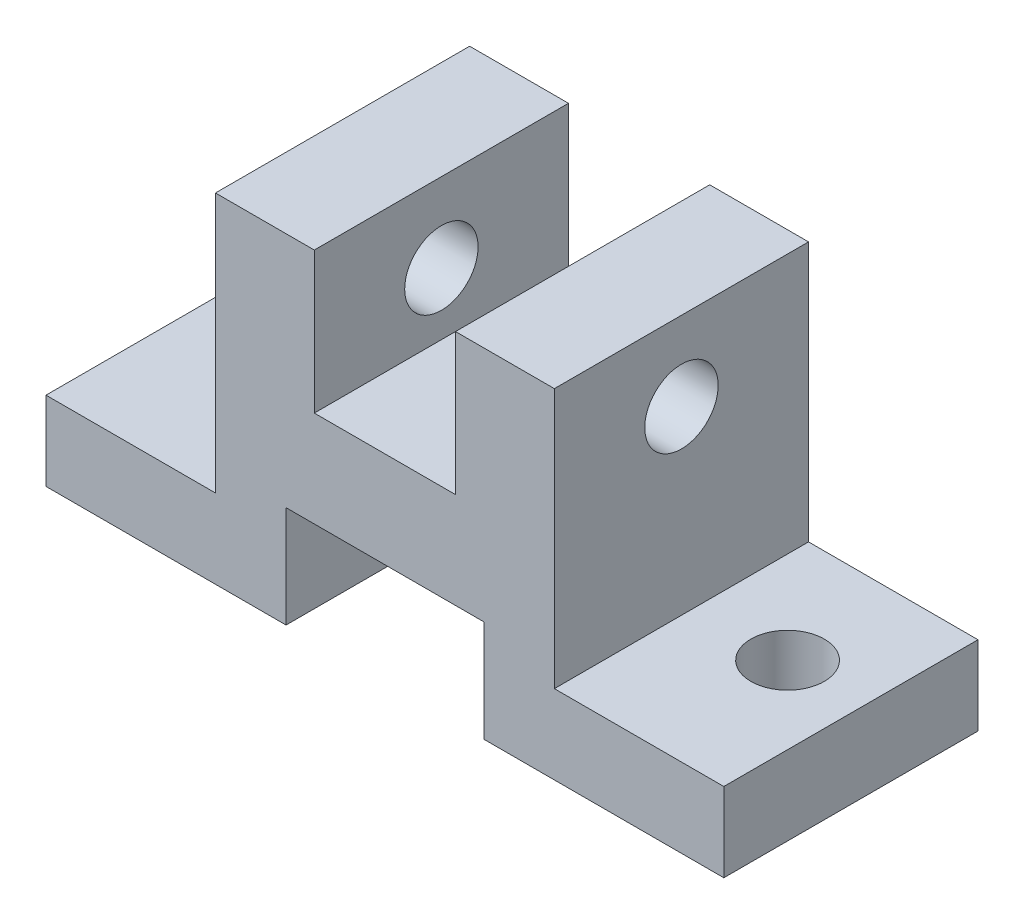
ISO-10303-21;
HEADER;
FILE_DESCRIPTION(('STEP AP214'),'2;1');
FILE_NAME('part.step','',(''),(''),'','','');
FILE_SCHEMA(('AUTOMOTIVE_DESIGN { 1 0 10303 214 1 1 1 1 }'));
ENDSEC;
DATA;
#1=APPLICATION_CONTEXT('core data for automotive mechanical design processes');
#2=APPLICATION_PROTOCOL_DEFINITION('international standard','automotive_design',2000,#1);
#3=PRODUCT_CONTEXT('',#1,'mechanical');
#4=PRODUCT('Part','Part','',(#3));
#5=PRODUCT_RELATED_PRODUCT_CATEGORY('part','',(#4));
#6=PRODUCT_DEFINITION_FORMATION('','',#4);
#7=PRODUCT_DEFINITION_CONTEXT('part definition',#1,'design');
#8=PRODUCT_DEFINITION('design','',#6,#7);
#9=PRODUCT_DEFINITION_SHAPE('','',#8);
#10=(LENGTH_UNIT() NAMED_UNIT(*) SI_UNIT(.MILLI.,.METRE.));
#11=(NAMED_UNIT(*) PLANE_ANGLE_UNIT() SI_UNIT($,.RADIAN.));
#12=(NAMED_UNIT(*) SI_UNIT($,.STERADIAN.) SOLID_ANGLE_UNIT());
#13=UNCERTAINTY_MEASURE_WITH_UNIT(LENGTH_MEASURE(1.E-05),#10,'distance_accuracy_value','');
#14=(GEOMETRIC_REPRESENTATION_CONTEXT(3) GLOBAL_UNCERTAINTY_ASSIGNED_CONTEXT((#13)) GLOBAL_UNIT_ASSIGNED_CONTEXT((#10,
#11,#12)) REPRESENTATION_CONTEXT('',''));
#15=CARTESIAN_POINT('',(0.,0.,0.));
#16=DIRECTION('',(0.,0.,1.));
#17=DIRECTION('',(1.,0.,0.));
#18=AXIS2_PLACEMENT_3D('',#15,#16,#17);
#19=CARTESIAN_POINT('',(0.,14.,45.));
#20=DIRECTION('',(1.,0.,0.));
#21=DIRECTION('',(0.,0.,-1.));
#22=AXIS2_PLACEMENT_3D('',#19,#20,#21);
#23=PLANE('',#22);
#24=DIRECTION('',(0.,-1.,0.));
#25=VECTOR('',#24,1.);
#26=CARTESIAN_POINT('',(0.,14.,0.));
#27=LINE('',#26,#25);
#28=CARTESIAN_POINT('',(0.,14.,0.));
#29=VERTEX_POINT('',#28);
#30=CARTESIAN_POINT('',(0.,0.,0.));
#31=VERTEX_POINT('',#30);
#32=EDGE_CURVE('E186',#29,#31,#27,.T.);
#33=ORIENTED_EDGE('',*,*,#32,.T.);
#34=DIRECTION('',(0.,0.,-1.));
#35=VECTOR('',#34,1.);
#36=CARTESIAN_POINT('',(0.,0.,45.));
#37=LINE('',#36,#35);
#38=CARTESIAN_POINT('',(0.,0.,45.));
#39=VERTEX_POINT('',#38);
#40=EDGE_CURVE('E11',#39,#31,#37,.T.);
#41=ORIENTED_EDGE('',*,*,#40,.F.);
#42=DIRECTION('',(0.,-1.,0.));
#43=VECTOR('',#42,1.);
#44=CARTESIAN_POINT('',(0.,14.,45.));
#45=LINE('',#44,#43);
#46=CARTESIAN_POINT('',(0.,14.,45.));
#47=VERTEX_POINT('',#46);
#48=EDGE_CURVE('E219',#47,#39,#45,.T.);
#49=ORIENTED_EDGE('',*,*,#48,.F.);
#50=DIRECTION('',(0.,0.,-1.));
#51=VECTOR('',#50,1.);
#52=CARTESIAN_POINT('',(0.,14.,45.));
#53=LINE('',#52,#51);
#54=EDGE_CURVE('E183',#47,#29,#53,.T.);
#55=ORIENTED_EDGE('',*,*,#54,.T.);
#56=EDGE_LOOP('',(#33,#41,#49,#55));
#57=FACE_BOUND('',#56,.T.);
#58=ADVANCED_FACE('F44',(#57),#23,.F.);
#59=CARTESIAN_POINT('',(0.,0.,45.));
#60=DIRECTION('',(0.,1.,0.));
#61=DIRECTION('',(0.,0.,1.));
#62=AXIS2_PLACEMENT_3D('',#59,#60,#61);
#63=PLANE('',#62);
#64=CARTESIAN_POINT('',(14.9196566145719,0.,20.));
#65=DIRECTION('',(0.,1.,0.));
#66=DIRECTION('',(0.,0.,1.));
#67=AXIS2_PLACEMENT_3D('',#64,#65,#66);
#68=CIRCLE('',#67,6.5);
#69=CARTESIAN_POINT('',(14.9196566145719,0.,26.5));
#70=VERTEX_POINT('',#69);
#71=EDGE_CURVE('E586',#70,#70,#68,.T.);
#72=ORIENTED_EDGE('',*,*,#71,.T.);
#73=EDGE_LOOP('',(#72));
#74=FACE_BOUND('',#73,.T.);
#75=DIRECTION('',(1.,0.,0.));
#76=VECTOR('',#75,1.);
#77=CARTESIAN_POINT('',(0.,0.,0.));
#78=LINE('',#77,#76);
#79=CARTESIAN_POINT('',(42.5,0.,0.));
#80=VERTEX_POINT('',#79);
#81=EDGE_CURVE('E195',#31,#80,#78,.T.);
#82=ORIENTED_EDGE('',*,*,#81,.T.);
#83=DIRECTION('',(0.,0.,-1.));
#84=VECTOR('',#83,1.);
#85=CARTESIAN_POINT('',(42.5,0.,45.));
#86=LINE('',#85,#84);
#87=CARTESIAN_POINT('',(42.5,0.,45.));
#88=VERTEX_POINT('',#87);
#89=EDGE_CURVE('E52',#88,#80,#86,.T.);
#90=ORIENTED_EDGE('',*,*,#89,.F.);
#91=DIRECTION('',(1.,0.,0.));
#92=VECTOR('',#91,1.);
#93=CARTESIAN_POINT('',(0.,0.,45.));
#94=LINE('',#93,#92);
#95=EDGE_CURVE('E126',#39,#88,#94,.T.);
#96=ORIENTED_EDGE('',*,*,#95,.F.);
#97=ORIENTED_EDGE('',*,*,#40,.T.);
#98=EDGE_LOOP('',(#82,#90,#96,#97));
#99=FACE_BOUND('',#98,.T.);
#100=ADVANCED_FACE('F321',(#74,#99),#63,.F.);
#101=CARTESIAN_POINT('',(42.5,0.,45.));
#102=DIRECTION('',(-1.,0.,0.));
#103=DIRECTION('',(0.,0.,1.));
#104=AXIS2_PLACEMENT_3D('',#101,#102,#103);
#105=PLANE('',#104);
#106=DIRECTION('',(0.,1.,0.));
#107=VECTOR('',#106,1.);
#108=CARTESIAN_POINT('',(42.5,0.,0.));
#109=LINE('',#108,#107);
#110=CARTESIAN_POINT('',(42.5,18.,0.));
#111=VERTEX_POINT('',#110);
#112=EDGE_CURVE('E192',#80,#111,#109,.T.);
#113=ORIENTED_EDGE('',*,*,#112,.T.);
#114=DIRECTION('',(0.,0.,-1.));
#115=VECTOR('',#114,1.);
#116=CARTESIAN_POINT('',(42.5,18.,45.));
#117=LINE('',#116,#115);
#118=CARTESIAN_POINT('',(42.5,18.,45.));
#119=VERTEX_POINT('',#118);
#120=EDGE_CURVE('E253',#119,#111,#117,.T.);
#121=ORIENTED_EDGE('',*,*,#120,.F.);
#122=DIRECTION('',(0.,1.,0.));
#123=VECTOR('',#122,1.);
#124=CARTESIAN_POINT('',(42.5,0.,45.));
#125=LINE('',#124,#123);
#126=EDGE_CURVE('E259',#88,#119,#125,.T.);
#127=ORIENTED_EDGE('',*,*,#126,.F.);
#128=ORIENTED_EDGE('',*,*,#89,.T.);
#129=EDGE_LOOP('',(#113,#121,#127,#128));
#130=FACE_BOUND('',#129,.T.);
#131=ADVANCED_FACE('F260',(#130),#105,.F.);
#132=CARTESIAN_POINT('',(42.5,18.,45.));
#133=DIRECTION('',(0.,1.,0.));
#134=DIRECTION('',(0.,0.,1.));
#135=AXIS2_PLACEMENT_3D('',#132,#133,#134);
#136=PLANE('',#135);
#137=DIRECTION('',(1.,0.,0.));
#138=VECTOR('',#137,1.);
#139=CARTESIAN_POINT('',(42.5,18.,0.));
#140=LINE('',#139,#138);
#141=CARTESIAN_POINT('',(77.5,18.,0.));
#142=VERTEX_POINT('',#141);
#143=EDGE_CURVE('E197',#111,#142,#140,.T.);
#144=ORIENTED_EDGE('',*,*,#143,.T.);
#145=DIRECTION('',(0.,0.,-1.));
#146=VECTOR('',#145,1.);
#147=CARTESIAN_POINT('',(77.5,18.,45.));
#148=LINE('',#147,#146);
#149=CARTESIAN_POINT('',(77.5,18.,45.));
#150=VERTEX_POINT('',#149);
#151=EDGE_CURVE('E246',#150,#142,#148,.T.);
#152=ORIENTED_EDGE('',*,*,#151,.F.);
#153=DIRECTION('',(1.,0.,0.));
#154=VECTOR('',#153,1.);
#155=CARTESIAN_POINT('',(42.5,18.,45.));
#156=LINE('',#155,#154);
#157=EDGE_CURVE('E280',#119,#150,#156,.T.);
#158=ORIENTED_EDGE('',*,*,#157,.F.);
#159=ORIENTED_EDGE('',*,*,#120,.T.);
#160=EDGE_LOOP('',(#144,#152,#158,#159));
#161=FACE_BOUND('',#160,.T.);
#162=ADVANCED_FACE('F268',(#161),#136,.F.);
#163=CARTESIAN_POINT('',(77.5,18.,45.));
#164=DIRECTION('',(1.,0.,0.));
#165=DIRECTION('',(0.,0.,-1.));
#166=AXIS2_PLACEMENT_3D('',#163,#164,#165);
#167=PLANE('',#166);
#168=DIRECTION('',(0.,-1.,0.));
#169=VECTOR('',#168,1.);
#170=CARTESIAN_POINT('',(77.5,18.,0.));
#171=LINE('',#170,#169);
#172=CARTESIAN_POINT('',(77.5,0.,0.));
#173=VERTEX_POINT('',#172);
#174=EDGE_CURVE('E200',#142,#173,#171,.T.);
#175=ORIENTED_EDGE('',*,*,#174,.T.);
#176=DIRECTION('',(0.,0.,-1.));
#177=VECTOR('',#176,1.);
#178=CARTESIAN_POINT('',(77.5,0.,45.));
#179=LINE('',#178,#177);
#180=CARTESIAN_POINT('',(77.5,0.,45.));
#181=VERTEX_POINT('',#180);
#182=EDGE_CURVE('E243',#181,#173,#179,.T.);
#183=ORIENTED_EDGE('',*,*,#182,.F.);
#184=DIRECTION('',(0.,-1.,0.));
#185=VECTOR('',#184,1.);
#186=CARTESIAN_POINT('',(77.5,18.,45.));
#187=LINE('',#186,#185);
#188=EDGE_CURVE('E273',#150,#181,#187,.T.);
#189=ORIENTED_EDGE('',*,*,#188,.F.);
#190=ORIENTED_EDGE('',*,*,#151,.T.);
#191=EDGE_LOOP('',(#175,#183,#189,#190));
#192=FACE_BOUND('',#191,.T.);
#193=ADVANCED_FACE('F275',(#192),#167,.F.);
#194=CARTESIAN_POINT('',(77.5,0.,45.));
#195=DIRECTION('',(0.,1.,0.));
#196=DIRECTION('',(0.,0.,1.));
#197=AXIS2_PLACEMENT_3D('',#194,#195,#196);
#198=PLANE('',#197);
#199=CARTESIAN_POINT('',(106.287852583252,0.,20.));
#200=DIRECTION('',(0.,1.,0.));
#201=DIRECTION('',(0.,0.,1.));
#202=AXIS2_PLACEMENT_3D('',#199,#200,#201);
#203=CIRCLE('',#202,6.5);
#204=CARTESIAN_POINT('',(106.287852583252,0.,26.5));
#205=VERTEX_POINT('',#204);
#206=EDGE_CURVE('E577',#205,#205,#203,.T.);
#207=ORIENTED_EDGE('',*,*,#206,.T.);
#208=EDGE_LOOP('',(#207));
#209=FACE_BOUND('',#208,.T.);
#210=DIRECTION('',(1.,0.,0.));
#211=VECTOR('',#210,1.);
#212=CARTESIAN_POINT('',(77.5,0.,0.));
#213=LINE('',#212,#211);
#214=CARTESIAN_POINT('',(120.,0.,0.));
#215=VERTEX_POINT('',#214);
#216=EDGE_CURVE('E203',#173,#215,#213,.T.);
#217=ORIENTED_EDGE('',*,*,#216,.T.);
#218=DIRECTION('',(0.,0.,-1.));
#219=VECTOR('',#218,1.);
#220=CARTESIAN_POINT('',(120.,0.,45.));
#221=LINE('',#220,#219);
#222=CARTESIAN_POINT('',(120.,0.,45.));
#223=VERTEX_POINT('',#222);
#224=EDGE_CURVE('E244',#223,#215,#221,.T.);
#225=ORIENTED_EDGE('',*,*,#224,.F.);
#226=DIRECTION('',(1.,0.,0.));
#227=VECTOR('',#226,1.);
#228=CARTESIAN_POINT('',(77.5,0.,45.));
#229=LINE('',#228,#227);
#230=EDGE_CURVE('E277',#181,#223,#229,.T.);
#231=ORIENTED_EDGE('',*,*,#230,.F.);
#232=ORIENTED_EDGE('',*,*,#182,.T.);
#233=EDGE_LOOP('',(#217,#225,#231,#232));
#234=FACE_BOUND('',#233,.T.);
#235=ADVANCED_FACE('F337',(#209,#234),#198,.F.);
#236=CARTESIAN_POINT('',(120.,0.,45.));
#237=DIRECTION('',(-1.,0.,0.));
#238=DIRECTION('',(0.,0.,1.));
#239=AXIS2_PLACEMENT_3D('',#236,#237,#238);
#240=PLANE('',#239);
#241=DIRECTION('',(0.,1.,0.));
#242=VECTOR('',#241,1.);
#243=CARTESIAN_POINT('',(120.,0.,0.));
#244=LINE('',#243,#242);
#245=CARTESIAN_POINT('',(120.,14.,0.));
#246=VERTEX_POINT('',#245);
#247=EDGE_CURVE('E201',#215,#246,#244,.T.);
#248=ORIENTED_EDGE('',*,*,#247,.T.);
#249=DIRECTION('',(0.,0.,-1.));
#250=VECTOR('',#249,1.);
#251=CARTESIAN_POINT('',(120.,14.,45.));
#252=LINE('',#251,#250);
#253=CARTESIAN_POINT('',(120.,14.,45.));
#254=VERTEX_POINT('',#253);
#255=EDGE_CURVE('E239',#254,#246,#252,.T.);
#256=ORIENTED_EDGE('',*,*,#255,.F.);
#257=DIRECTION('',(0.,1.,0.));
#258=VECTOR('',#257,1.);
#259=CARTESIAN_POINT('',(120.,0.,45.));
#260=LINE('',#259,#258);
#261=EDGE_CURVE('E276',#223,#254,#260,.T.);
#262=ORIENTED_EDGE('',*,*,#261,.F.);
#263=ORIENTED_EDGE('',*,*,#224,.T.);
#264=EDGE_LOOP('',(#248,#256,#262,#263));
#265=FACE_BOUND('',#264,.T.);
#266=ADVANCED_FACE('F336',(#265),#240,.F.);
#267=CARTESIAN_POINT('',(120.,14.,45.));
#268=DIRECTION('',(0.,-1.,0.));
#269=DIRECTION('',(0.,0.,-1.));
#270=AXIS2_PLACEMENT_3D('',#267,#268,#269);
#271=PLANE('',#270);
#272=CARTESIAN_POINT('',(106.287852583252,14.,20.));
#273=DIRECTION('',(0.,1.,0.));
#274=DIRECTION('',(0.,0.,1.));
#275=AXIS2_PLACEMENT_3D('',#272,#273,#274);
#276=CIRCLE('',#275,6.5);
#277=CARTESIAN_POINT('',(106.287852583252,14.,26.5));
#278=VERTEX_POINT('',#277);
#279=EDGE_CURVE('E581',#278,#278,#276,.T.);
#280=ORIENTED_EDGE('',*,*,#279,.F.);
#281=EDGE_LOOP('',(#280));
#282=FACE_BOUND('',#281,.T.);
#283=DIRECTION('',(-1.,0.,0.));
#284=VECTOR('',#283,1.);
#285=CARTESIAN_POINT('',(120.,14.,0.));
#286=LINE('',#285,#284);
#287=CARTESIAN_POINT('',(90.,14.,0.));
#288=VERTEX_POINT('',#287);
#289=EDGE_CURVE('E202',#246,#288,#286,.T.);
#290=ORIENTED_EDGE('',*,*,#289,.T.);
#291=DIRECTION('',(0.,0.,-1.));
#292=VECTOR('',#291,1.);
#293=CARTESIAN_POINT('',(90.,14.,45.));
#294=LINE('',#293,#292);
#295=CARTESIAN_POINT('',(90.,14.,45.));
#296=VERTEX_POINT('',#295);
#297=EDGE_CURVE('E237',#296,#288,#294,.T.);
#298=ORIENTED_EDGE('',*,*,#297,.F.);
#299=DIRECTION('',(-1.,0.,0.));
#300=VECTOR('',#299,1.);
#301=CARTESIAN_POINT('',(120.,14.,45.));
#302=LINE('',#301,#300);
#303=EDGE_CURVE('E283',#254,#296,#302,.T.);
#304=ORIENTED_EDGE('',*,*,#303,.F.);
#305=ORIENTED_EDGE('',*,*,#255,.T.);
#306=EDGE_LOOP('',(#290,#298,#304,#305));
#307=FACE_BOUND('',#306,.T.);
#308=ADVANCED_FACE('F341',(#282,#307),#271,.F.);
#309=CARTESIAN_POINT('',(90.,14.,45.));
#310=DIRECTION('',(-1.,0.,0.));
#311=DIRECTION('',(0.,0.,1.));
#312=AXIS2_PLACEMENT_3D('',#309,#310,#311);
#313=PLANE('',#312);
#314=CARTESIAN_POINT('',(90.,46.,22.5));
#315=DIRECTION('',(1.,0.,0.));
#316=DIRECTION('',(0.,0.,-1.));
#317=AXIS2_PLACEMENT_3D('',#314,#315,#316);
#318=CIRCLE('',#317,6.5);
#319=CARTESIAN_POINT('',(90.,46.,16.));
#320=VERTEX_POINT('',#319);
#321=EDGE_CURVE('E587',#320,#320,#318,.T.);
#322=ORIENTED_EDGE('',*,*,#321,.F.);
#323=EDGE_LOOP('',(#322));
#324=FACE_BOUND('',#323,.T.);
#325=DIRECTION('',(0.,1.,0.));
#326=VECTOR('',#325,1.);
#327=CARTESIAN_POINT('',(90.,14.,0.));
#328=LINE('',#327,#326);
#329=CARTESIAN_POINT('',(90.,60.,0.));
#330=VERTEX_POINT('',#329);
#331=EDGE_CURVE('E210',#288,#330,#328,.T.);
#332=ORIENTED_EDGE('',*,*,#331,.T.);
#333=DIRECTION('',(0.,0.,-1.));
#334=VECTOR('',#333,1.);
#335=CARTESIAN_POINT('',(90.,60.,45.));
#336=LINE('',#335,#334);
#337=CARTESIAN_POINT('',(90.,60.,45.));
#338=VERTEX_POINT('',#337);
#339=EDGE_CURVE('E231',#338,#330,#336,.T.);
#340=ORIENTED_EDGE('',*,*,#339,.F.);
#341=DIRECTION('',(0.,1.,0.));
#342=VECTOR('',#341,1.);
#343=CARTESIAN_POINT('',(90.,14.,45.));
#344=LINE('',#343,#342);
#345=EDGE_CURVE('E290',#296,#338,#344,.T.);
#346=ORIENTED_EDGE('',*,*,#345,.F.);
#347=ORIENTED_EDGE('',*,*,#297,.T.);
#348=EDGE_LOOP('',(#332,#340,#346,#347));
#349=FACE_BOUND('',#348,.T.);
#350=ADVANCED_FACE('F350',(#324,#349),#313,.F.);
#351=CARTESIAN_POINT('',(90.,60.,45.));
#352=DIRECTION('',(0.,-1.,0.));
#353=DIRECTION('',(0.,0.,-1.));
#354=AXIS2_PLACEMENT_3D('',#351,#352,#353);
#355=PLANE('',#354);
#356=DIRECTION('',(-1.,0.,0.));
#357=VECTOR('',#356,1.);
#358=CARTESIAN_POINT('',(90.,60.,0.));
#359=LINE('',#358,#357);
#360=CARTESIAN_POINT('',(72.5,60.,0.));
#361=VERTEX_POINT('',#360);
#362=EDGE_CURVE('E207',#330,#361,#359,.T.);
#363=ORIENTED_EDGE('',*,*,#362,.T.);
#364=DIRECTION('',(0.,0.,-1.));
#365=VECTOR('',#364,1.);
#366=CARTESIAN_POINT('',(72.5,60.,45.));
#367=LINE('',#366,#365);
#368=CARTESIAN_POINT('',(72.5,60.,45.));
#369=VERTEX_POINT('',#368);
#370=EDGE_CURVE('E228',#369,#361,#367,.T.);
#371=ORIENTED_EDGE('',*,*,#370,.F.);
#372=DIRECTION('',(-1.,0.,0.));
#373=VECTOR('',#372,1.);
#374=CARTESIAN_POINT('',(90.,60.,45.));
#375=LINE('',#374,#373);
#376=EDGE_CURVE('E289',#338,#369,#375,.T.);
#377=ORIENTED_EDGE('',*,*,#376,.F.);
#378=ORIENTED_EDGE('',*,*,#339,.T.);
#379=EDGE_LOOP('',(#363,#371,#377,#378));
#380=FACE_BOUND('',#379,.T.);
#381=ADVANCED_FACE('F352',(#380),#355,.F.);
#382=CARTESIAN_POINT('',(72.5,60.,45.));
#383=DIRECTION('',(1.,0.,0.));
#384=DIRECTION('',(0.,0.,-1.));
#385=AXIS2_PLACEMENT_3D('',#382,#383,#384);
#386=PLANE('',#385);
#387=CARTESIAN_POINT('',(72.5,46.,22.5));
#388=DIRECTION('',(1.,0.,0.));
#389=DIRECTION('',(0.,0.,-1.));
#390=AXIS2_PLACEMENT_3D('',#387,#388,#389);
#391=CIRCLE('',#390,6.5);
#392=CARTESIAN_POINT('',(72.5,46.,16.));
#393=VERTEX_POINT('',#392);
#394=EDGE_CURVE('E593',#393,#393,#391,.T.);
#395=ORIENTED_EDGE('',*,*,#394,.T.);
#396=EDGE_LOOP('',(#395));
#397=FACE_BOUND('',#396,.T.);
#398=DIRECTION('',(0.,-1.,0.));
#399=VECTOR('',#398,1.);
#400=CARTESIAN_POINT('',(72.5,60.,0.));
#401=LINE('',#400,#399);
#402=CARTESIAN_POINT('',(72.5,35.,0.));
#403=VERTEX_POINT('',#402);
#404=EDGE_CURVE('E211',#361,#403,#401,.T.);
#405=ORIENTED_EDGE('',*,*,#404,.T.);
#406=DIRECTION('',(0.,0.,-1.));
#407=VECTOR('',#406,1.);
#408=CARTESIAN_POINT('',(72.5,35.,45.));
#409=LINE('',#408,#407);
#410=CARTESIAN_POINT('',(72.5,35.,45.));
#411=VERTEX_POINT('',#410);
#412=EDGE_CURVE('E229',#411,#403,#409,.T.);
#413=ORIENTED_EDGE('',*,*,#412,.F.);
#414=DIRECTION('',(0.,-1.,0.));
#415=VECTOR('',#414,1.);
#416=CARTESIAN_POINT('',(72.5,60.,45.));
#417=LINE('',#416,#415);
#418=EDGE_CURVE('E292',#369,#411,#417,.T.);
#419=ORIENTED_EDGE('',*,*,#418,.F.);
#420=ORIENTED_EDGE('',*,*,#370,.T.);
#421=EDGE_LOOP('',(#405,#413,#419,#420));
#422=FACE_BOUND('',#421,.T.);
#423=ADVANCED_FACE('F353',(#397,#422),#386,.F.);
#424=CARTESIAN_POINT('',(72.5,35.,45.));
#425=DIRECTION('',(0.,-1.,0.));
#426=DIRECTION('',(0.,0.,-1.));
#427=AXIS2_PLACEMENT_3D('',#424,#425,#426);
#428=PLANE('',#427);
#429=DIRECTION('',(-1.,0.,0.));
#430=VECTOR('',#429,1.);
#431=CARTESIAN_POINT('',(72.5,35.,0.));
#432=LINE('',#431,#430);
#433=CARTESIAN_POINT('',(47.5,35.,0.));
#434=VERTEX_POINT('',#433);
#435=EDGE_CURVE('E213',#403,#434,#432,.T.);
#436=ORIENTED_EDGE('',*,*,#435,.T.);
#437=DIRECTION('',(0.,0.,-1.));
#438=VECTOR('',#437,1.);
#439=CARTESIAN_POINT('',(47.5,35.,45.));
#440=LINE('',#439,#438);
#441=CARTESIAN_POINT('',(47.5,35.,45.));
#442=VERTEX_POINT('',#441);
#443=EDGE_CURVE('E221',#442,#434,#440,.T.);
#444=ORIENTED_EDGE('',*,*,#443,.F.);
#445=DIRECTION('',(-1.,0.,0.));
#446=VECTOR('',#445,1.);
#447=CARTESIAN_POINT('',(72.5,35.,45.));
#448=LINE('',#447,#446);
#449=EDGE_CURVE('E291',#411,#442,#448,.T.);
#450=ORIENTED_EDGE('',*,*,#449,.F.);
#451=ORIENTED_EDGE('',*,*,#412,.T.);
#452=EDGE_LOOP('',(#436,#444,#450,#451));
#453=FACE_BOUND('',#452,.T.);
#454=ADVANCED_FACE('F296',(#453),#428,.F.);
#455=CARTESIAN_POINT('',(47.5,35.,45.));
#456=DIRECTION('',(-1.,0.,0.));
#457=DIRECTION('',(0.,0.,1.));
#458=AXIS2_PLACEMENT_3D('',#455,#456,#457);
#459=PLANE('',#458);
#460=CARTESIAN_POINT('',(47.5,46.,22.5));
#461=DIRECTION('',(-1.,0.,0.));
#462=DIRECTION('',(0.,0.,1.));
#463=AXIS2_PLACEMENT_3D('',#460,#461,#462);
#464=CIRCLE('',#463,6.5);
#465=CARTESIAN_POINT('',(47.5,46.,29.));
#466=VERTEX_POINT('',#465);
#467=EDGE_CURVE('E191',#466,#466,#464,.T.);
#468=ORIENTED_EDGE('',*,*,#467,.T.);
#469=EDGE_LOOP('',(#468));
#470=FACE_BOUND('',#469,.T.);
#471=DIRECTION('',(0.,1.,0.));
#472=VECTOR('',#471,1.);
#473=CARTESIAN_POINT('',(47.5,35.,0.));
#474=LINE('',#473,#472);
#475=CARTESIAN_POINT('',(47.5,60.,0.));
#476=VERTEX_POINT('',#475);
#477=EDGE_CURVE('E214',#434,#476,#474,.T.);
#478=ORIENTED_EDGE('',*,*,#477,.T.);
#479=DIRECTION('',(0.,0.,-1.));
#480=VECTOR('',#479,1.);
#481=CARTESIAN_POINT('',(47.5,60.,45.));
#482=LINE('',#481,#480);
#483=CARTESIAN_POINT('',(47.5,60.,45.));
#484=VERTEX_POINT('',#483);
#485=EDGE_CURVE('E177',#484,#476,#482,.T.);
#486=ORIENTED_EDGE('',*,*,#485,.F.);
#487=DIRECTION('',(0.,1.,0.));
#488=VECTOR('',#487,1.);
#489=CARTESIAN_POINT('',(47.5,35.,45.));
#490=LINE('',#489,#488);
#491=EDGE_CURVE('E172',#442,#484,#490,.T.);
#492=ORIENTED_EDGE('',*,*,#491,.F.);
#493=ORIENTED_EDGE('',*,*,#443,.T.);
#494=EDGE_LOOP('',(#478,#486,#492,#493));
#495=FACE_BOUND('',#494,.T.);
#496=ADVANCED_FACE('F301',(#470,#495),#459,.F.);
#497=CARTESIAN_POINT('',(47.5,60.,45.));
#498=DIRECTION('',(0.,-1.,0.));
#499=DIRECTION('',(0.,0.,-1.));
#500=AXIS2_PLACEMENT_3D('',#497,#498,#499);
#501=PLANE('',#500);
#502=DIRECTION('',(-1.,0.,0.));
#503=VECTOR('',#502,1.);
#504=CARTESIAN_POINT('',(47.5,60.,0.));
#505=LINE('',#504,#503);
#506=CARTESIAN_POINT('',(30.,60.,0.));
#507=VERTEX_POINT('',#506);
#508=EDGE_CURVE('E179',#476,#507,#505,.T.);
#509=ORIENTED_EDGE('',*,*,#508,.T.);
#510=DIRECTION('',(0.,0.,-1.));
#511=VECTOR('',#510,1.);
#512=CARTESIAN_POINT('',(30.,60.,45.));
#513=LINE('',#512,#511);
#514=CARTESIAN_POINT('',(30.,60.,45.));
#515=VERTEX_POINT('',#514);
#516=EDGE_CURVE('E178',#515,#507,#513,.T.);
#517=ORIENTED_EDGE('',*,*,#516,.F.);
#518=DIRECTION('',(-1.,0.,0.));
#519=VECTOR('',#518,1.);
#520=CARTESIAN_POINT('',(47.5,60.,45.));
#521=LINE('',#520,#519);
#522=EDGE_CURVE('E164',#484,#515,#521,.T.);
#523=ORIENTED_EDGE('',*,*,#522,.F.);
#524=ORIENTED_EDGE('',*,*,#485,.T.);
#525=EDGE_LOOP('',(#509,#517,#523,#524));
#526=FACE_BOUND('',#525,.T.);
#527=ADVANCED_FACE('F180',(#526),#501,.F.);
#528=CARTESIAN_POINT('',(30.,60.,45.));
#529=DIRECTION('',(1.,0.,0.));
#530=DIRECTION('',(0.,0.,-1.));
#531=AXIS2_PLACEMENT_3D('',#528,#529,#530);
#532=PLANE('',#531);
#533=CARTESIAN_POINT('',(30.,46.,22.5));
#534=DIRECTION('',(-1.,0.,0.));
#535=DIRECTION('',(0.,0.,1.));
#536=AXIS2_PLACEMENT_3D('',#533,#534,#535);
#537=CIRCLE('',#536,6.5);
#538=CARTESIAN_POINT('',(30.,46.,29.));
#539=VERTEX_POINT('',#538);
#540=EDGE_CURVE('E596',#539,#539,#537,.T.);
#541=ORIENTED_EDGE('',*,*,#540,.F.);
#542=EDGE_LOOP('',(#541));
#543=FACE_BOUND('',#542,.T.);
#544=DIRECTION('',(0.,-1.,0.));
#545=VECTOR('',#544,1.);
#546=CARTESIAN_POINT('',(30.,60.,0.));
#547=LINE('',#546,#545);
#548=CARTESIAN_POINT('',(30.,14.,0.));
#549=VERTEX_POINT('',#548);
#550=EDGE_CURVE('E111',#507,#549,#547,.T.);
#551=ORIENTED_EDGE('',*,*,#550,.T.);
#552=DIRECTION('',(0.,0.,-1.));
#553=VECTOR('',#552,1.);
#554=CARTESIAN_POINT('',(30.,14.,45.));
#555=LINE('',#554,#553);
#556=CARTESIAN_POINT('',(30.,14.,45.));
#557=VERTEX_POINT('',#556);
#558=EDGE_CURVE('E182',#557,#549,#555,.T.);
#559=ORIENTED_EDGE('',*,*,#558,.F.);
#560=DIRECTION('',(0.,-1.,0.));
#561=VECTOR('',#560,1.);
#562=CARTESIAN_POINT('',(30.,60.,45.));
#563=LINE('',#562,#561);
#564=EDGE_CURVE('E166',#515,#557,#563,.T.);
#565=ORIENTED_EDGE('',*,*,#564,.F.);
#566=ORIENTED_EDGE('',*,*,#516,.T.);
#567=EDGE_LOOP('',(#551,#559,#565,#566));
#568=FACE_BOUND('',#567,.T.);
#569=ADVANCED_FACE('F181',(#543,#568),#532,.F.);
#570=CARTESIAN_POINT('',(30.,14.,45.));
#571=DIRECTION('',(0.,-1.,0.));
#572=DIRECTION('',(0.,0.,-1.));
#573=AXIS2_PLACEMENT_3D('',#570,#571,#572);
#574=PLANE('',#573);
#575=CARTESIAN_POINT('',(14.9196566145719,14.,20.));
#576=DIRECTION('',(0.,1.,0.));
#577=DIRECTION('',(0.,0.,1.));
#578=AXIS2_PLACEMENT_3D('',#575,#576,#577);
#579=CIRCLE('',#578,6.5);
#580=CARTESIAN_POINT('',(14.9196566145719,14.,26.5));
#581=VERTEX_POINT('',#580);
#582=EDGE_CURVE('E584',#581,#581,#579,.T.);
#583=ORIENTED_EDGE('',*,*,#582,.F.);
#584=EDGE_LOOP('',(#583));
#585=FACE_BOUND('',#584,.T.);
#586=DIRECTION('',(-1.,0.,0.));
#587=VECTOR('',#586,1.);
#588=CARTESIAN_POINT('',(30.,14.,0.));
#589=LINE('',#588,#587);
#590=EDGE_CURVE('E118',#549,#29,#589,.T.);
#591=ORIENTED_EDGE('',*,*,#590,.T.);
#592=ORIENTED_EDGE('',*,*,#54,.F.);
#593=DIRECTION('',(-1.,0.,0.));
#594=VECTOR('',#593,1.);
#595=CARTESIAN_POINT('',(30.,14.,45.));
#596=LINE('',#595,#594);
#597=EDGE_CURVE('E62',#557,#47,#596,.T.);
#598=ORIENTED_EDGE('',*,*,#597,.F.);
#599=ORIENTED_EDGE('',*,*,#558,.T.);
#600=EDGE_LOOP('',(#591,#592,#598,#599));
#601=FACE_BOUND('',#600,.T.);
#602=ADVANCED_FACE('F307',(#585,#601),#574,.F.);
#603=CARTESIAN_POINT('',(0.,0.,45.));
#604=DIRECTION('',(0.,0.,1.));
#605=DIRECTION('',(1.,0.,0.));
#606=AXIS2_PLACEMENT_3D('',#603,#604,#605);
#607=PLANE('',#606);
#608=ORIENTED_EDGE('',*,*,#48,.T.);
#609=ORIENTED_EDGE('',*,*,#95,.T.);
#610=ORIENTED_EDGE('',*,*,#126,.T.);
#611=ORIENTED_EDGE('',*,*,#157,.T.);
#612=ORIENTED_EDGE('',*,*,#188,.T.);
#613=ORIENTED_EDGE('',*,*,#230,.T.);
#614=ORIENTED_EDGE('',*,*,#261,.T.);
#615=ORIENTED_EDGE('',*,*,#303,.T.);
#616=ORIENTED_EDGE('',*,*,#345,.T.);
#617=ORIENTED_EDGE('',*,*,#376,.T.);
#618=ORIENTED_EDGE('',*,*,#418,.T.);
#619=ORIENTED_EDGE('',*,*,#449,.T.);
#620=ORIENTED_EDGE('',*,*,#491,.T.);
#621=ORIENTED_EDGE('',*,*,#522,.T.);
#622=ORIENTED_EDGE('',*,*,#564,.T.);
#623=ORIENTED_EDGE('',*,*,#597,.T.);
#624=EDGE_LOOP('',(#608,#609,#610,#611,#612,#613,#614,#615,#616,#617,#618,#619,#620,#621,#622,#623));
#625=FACE_BOUND('',#624,.T.);
#626=ADVANCED_FACE('F170',(#625),#607,.T.);
#627=CARTESIAN_POINT('',(0.,0.,0.));
#628=DIRECTION('',(0.,0.,1.));
#629=DIRECTION('',(1.,0.,0.));
#630=AXIS2_PLACEMENT_3D('',#627,#628,#629);
#631=PLANE('',#630);
#632=ORIENTED_EDGE('',*,*,#32,.F.);
#633=ORIENTED_EDGE('',*,*,#590,.F.);
#634=ORIENTED_EDGE('',*,*,#550,.F.);
#635=ORIENTED_EDGE('',*,*,#508,.F.);
#636=ORIENTED_EDGE('',*,*,#477,.F.);
#637=ORIENTED_EDGE('',*,*,#435,.F.);
#638=ORIENTED_EDGE('',*,*,#404,.F.);
#639=ORIENTED_EDGE('',*,*,#362,.F.);
#640=ORIENTED_EDGE('',*,*,#331,.F.);
#641=ORIENTED_EDGE('',*,*,#289,.F.);
#642=ORIENTED_EDGE('',*,*,#247,.F.);
#643=ORIENTED_EDGE('',*,*,#216,.F.);
#644=ORIENTED_EDGE('',*,*,#174,.F.);
#645=ORIENTED_EDGE('',*,*,#143,.F.);
#646=ORIENTED_EDGE('',*,*,#112,.F.);
#647=ORIENTED_EDGE('',*,*,#81,.F.);
#648=EDGE_LOOP('',(#632,#633,#634,#635,#636,#637,#638,#639,#640,#641,#642,#643,#644,#645,#646,#647));
#649=FACE_BOUND('',#648,.T.);
#650=ADVANCED_FACE('F263',(#649),#631,.F.);
#651=CARTESIAN_POINT('',(47.5,46.,22.5));
#652=DIRECTION('',(-1.,0.,0.));
#653=DIRECTION('',(0.,0.,1.));
#654=AXIS2_PLACEMENT_3D('',#651,#652,#653);
#655=CYLINDRICAL_SURFACE('',#654,6.5);
#656=ORIENTED_EDGE('',*,*,#467,.F.);
#657=EDGE_LOOP('',(#656));
#658=FACE_BOUND('',#657,.T.);
#659=ORIENTED_EDGE('',*,*,#540,.T.);
#660=EDGE_LOOP('',(#659));
#661=FACE_BOUND('',#660,.T.);
#662=ADVANCED_FACE('F398',(#658,#661),#655,.F.);
#663=CARTESIAN_POINT('',(72.5,46.,22.5));
#664=DIRECTION('',(1.,0.,0.));
#665=DIRECTION('',(0.,0.,-1.));
#666=AXIS2_PLACEMENT_3D('',#663,#664,#665);
#667=CYLINDRICAL_SURFACE('',#666,6.5);
#668=ORIENTED_EDGE('',*,*,#394,.F.);
#669=EDGE_LOOP('',(#668));
#670=FACE_BOUND('',#669,.T.);
#671=ORIENTED_EDGE('',*,*,#321,.T.);
#672=EDGE_LOOP('',(#671));
#673=FACE_BOUND('',#672,.T.);
#674=ADVANCED_FACE('F548',(#670,#673),#667,.F.);
#675=CARTESIAN_POINT('',(14.9196566145719,0.,20.));
#676=DIRECTION('',(0.,1.,0.));
#677=DIRECTION('',(0.,0.,1.));
#678=AXIS2_PLACEMENT_3D('',#675,#676,#677);
#679=CYLINDRICAL_SURFACE('',#678,6.5);
#680=ORIENTED_EDGE('',*,*,#71,.F.);
#681=EDGE_LOOP('',(#680));
#682=FACE_BOUND('',#681,.T.);
#683=ORIENTED_EDGE('',*,*,#582,.T.);
#684=EDGE_LOOP('',(#683));
#685=FACE_BOUND('',#684,.T.);
#686=ADVANCED_FACE('F559',(#682,#685),#679,.F.);
#687=CARTESIAN_POINT('',(106.287852583252,0.,20.));
#688=DIRECTION('',(0.,1.,0.));
#689=DIRECTION('',(0.,0.,1.));
#690=AXIS2_PLACEMENT_3D('',#687,#688,#689);
#691=CYLINDRICAL_SURFACE('',#690,6.5);
#692=ORIENTED_EDGE('',*,*,#206,.F.);
#693=EDGE_LOOP('',(#692));
#694=FACE_BOUND('',#693,.T.);
#695=ORIENTED_EDGE('',*,*,#279,.T.);
#696=EDGE_LOOP('',(#695));
#697=FACE_BOUND('',#696,.T.);
#698=ADVANCED_FACE('F562',(#694,#697),#691,.F.);
#699=CLOSED_SHELL('',(#58,#100,#131,#162,#193,#235,#266,#308,#350,#381,#423,#454,#496,#527,#569,
#602,#626,#650,#662,#674,#686,#698));
#700=MANIFOLD_SOLID_BREP('B2',#699);
#701=ADVANCED_BREP_SHAPE_REPRESENTATION('',(#18,#700),#14);
#702=SHAPE_DEFINITION_REPRESENTATION(#9,#701);
ENDSEC;
END-ISO-10303-21;
